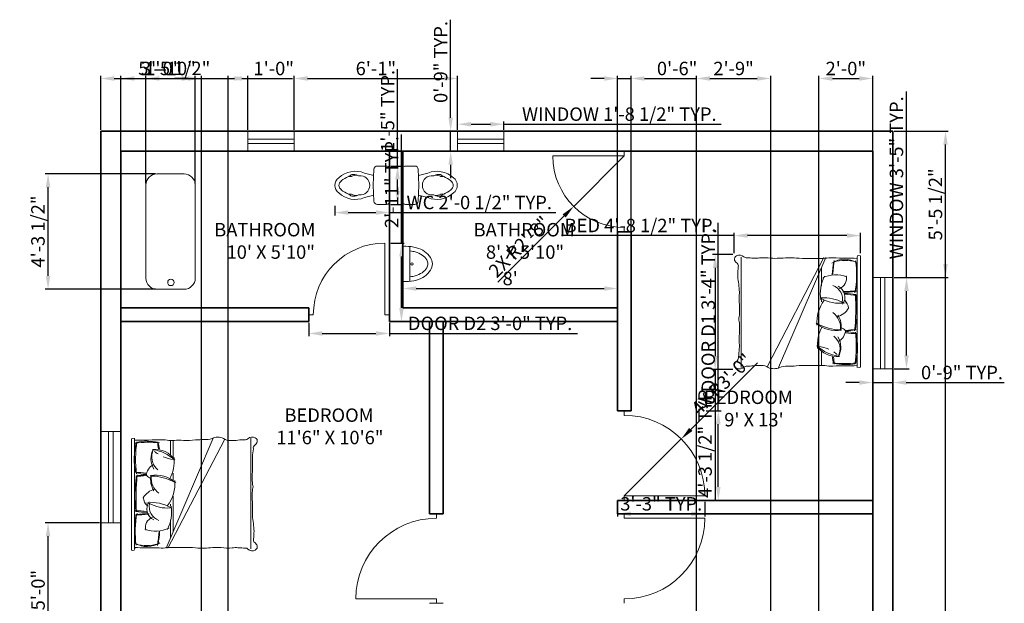
# Model space of a CAD drawing. Units: inches. Extents: x 88375 to 88815, y 24230 to 25146.
# Tile 2 of 3: x 88375 to 88815, y 24513 to 24774. Entities that reach past the tile are written whole.
import ezdxf

# ---------------------------------------------------------------- set-up
doc = ezdxf.new("R2010")
doc.units = ezdxf.units.IN
for name, color, linetype, lineweight in [('A-ANNO-DIMS', 2, 'Continuous', 18), ('A-AREA-IDEN', 7, 'Continuous', 18), ('A-WALL', 7, 'Continuous', 35), ('doors', 50, 'Continuous', 18), ('SANTEH', 5, 'Continuous', 18), ('windows', 70, 'Continuous', 18)]:
    doc.layers.add(name, color=color, linetype=linetype, lineweight=lineweight)
doc.layers.add('A-FURN', color=141, linetype='Continuous', lineweight=18, true_color=0xadddf7)
doc.styles.get("Standard").update_dxf_attribs({"font": 'arial.ttf'})
doc.dimstyles.new('ISO-25', dxfattribs={"dimtxt": 6, "dimasz": 6, "dimexe": 1.25, "dimexo": 0.625, "dimtad": 1, "dimdec": 0, "dimlunit": 3, "dimtxsty": 'Standard', "dimcen": 2.5, "dimclrd": 1, "dimclre": 1, "dimclrt": 2, "dimadec": 0, "dimazin": 0, "dimtfac": 1, "dimtdec": 0, "dimtmove": 0, "dimatfit": 3, "dimfxl": 1, "dimarcsym": 0})

# ---------------------------------------------------------------- blocks, each defined once
blk = doc.blocks.new('*D1')
at = {"layer": 'A-ANNO-DIMS', "color": 0, "lineweight": -2, "transparency": 16777216}
for p, q in [((88546.55, 24652.53), (88546.55, 24654.95)), ((88552.55, 24653.7), (88636.55, 24653.7)), ((88642.55, 24652.53), (88642.55, 24654.95))]:
    blk.add_line(p, q, dxfattribs=at)
at = {"layer": 'A-ANNO-DIMS', "color": 0, "transparency": 16777216}
for points in [[(88552.55, 24654.7), (88552.55, 24652.7), (88546.55, 24653.7)], [(88636.55, 24654.7), (88636.55, 24652.7), (88642.55, 24653.7)]]:
    blk.add_solid(points, dxfattribs=at)
at = {"layer": 'Defpoints', "color": 0, "transparency": 16777216}
for p in [(88546.55, 24651.91), (88642.55, 24653.7), (88642.55, 24651.91)]:
    blk.add_point(p, dxfattribs=at)
at = {"layer": 'A-ANNO-DIMS', "color": 0, "transparency": 16777216, "insert": (88594.55, 24657.39), "char_height": 6, "attachment_point": 5}
blk.add_mtext("8'", dxfattribs=at)
blk = doc.blocks.new('BED-DOUBLE-PLAN')
for p, q in [((1.4, 0.9), (1.4, 50.31)), ((15.52, 1.15), (36.6, 50.31)), ((16.31, 1.15), (41.56, 49.64)), ((17.42, 42.88), (17.42, 49.34)), ((18.75, 41.86), (18.75, 49.34)), ((53.33, 0.9), (53.33, 50.31)), ((18.75, 31.74), (18.75, 34.71)), ((18.75, 8.33), (18.75, 24.37)), ((17.42, 19.9), (17.42, 20.88)), ((17.42, 5.64), (17.42, 13.88))]:
    blk.add_line(p, q)
blk.add_lwpolyline([(1.54, 49.41, 0.098699), (1.25, 50.08, 0.222522), (0, 50.08), (0, 0.33, 0.171621), (1.3, 0.3, 0.102495), (1.54, 1.48, 0.015571), (6.35, 1.41, 0.00267), (12.35, 1.29, 0.058958), (15.95, 1.46, -0.038458), (19.2, 1.53, 0.025508), (23.25, 1.53, -0.039412), (28.66, 1.33, 0.016498), (32.6, 1.18, -0.035771), (40.08, 1.43, 0.045388), (45.04, 1.29, -0.080578), (47.62, 1.41, 0.026504), (50.99, 1.23, -0.211134), (52.07, 0.79, 0.329446), (55.35, 0.34, 0.37589), (56.22, 2.29, 0.123892), (55.14, 3.69, -0.342539), (54.6, 5.33, 0.07104), (54.53, 12.17, -0.036442), (54.14, 15.72, -0.046791), (54.19, 18.58, 0.023628), (54.14, 21.2, -0.055897), (54.2, 27.56, 0.053528), (54.38, 28.63, 0.053528), (54.2, 29.69, -0.055897), (54.14, 36.05, 0.026973), (54.19, 38.35, -0.036947), (54.14, 41.97, -0.036442), (54.53, 45.52, -0.281256), (55.14, 47.2, -0.521995), (55.14, 47.2, 0.123892), (56.22, 48.6, 0.37589), (55.35, 50.55, 0.329446), (52.07, 50.1, -0.211134), (50.99, 49.66, 0.026504), (47.62, 49.48, -0.06219), (44.27, 49.36, -0.218233), (41.22, 50.22, 0.123513), (38.6, 50.78, 0.129887), (36.08, 50.23, -0.095063), (32.6, 49.71, 0.016498), (28.66, 49.56, -0.039412), (23.25, 49.36, 0.025508), (19.2, 49.36, -0.038458), (15.95, 49.43, 0.058958), (12.35, 49.6, 0.00267), (6.35, 49.48, 0.015571)], format="xyb", close=True)
for centre, radius, start, end in [((28.69, 41.4), 27.41, 165.0181, 193.7392), ((7.34, -1.74), 50.25, 84.0935, 96.4707), ((54.72, 40.85), 52.84, 171.3714, 186.917), ((6.88, 26.06), 22.91, 77.3175, 101.7435), ((30.71, 48.94), 18.95, 180.6432, 190.2707), ((-1.93, 44.06), 14.51, 5.447, 17.4199), ((17.81, 41.21), 9.06, 151.6404, 211.3345), ((16.4, 41.97), 7.31, 151.8876, 231.8707), ((10.64, 34.91), 10.43, 32.3262, 97), ((7.31, 27.91), 17.47, 47.3201, 81.4624), ((20.44, 56.37), 15.6, 229.9508, 236.951), ((20.44, 56.37), 15.6, 246.2982, 263.8539), ((2.46, 40.16), 16.73, 330.9467, 5.467), ((12.85, 33.14), 6.24, 118.1996, 176.5061), ((56.67, 24.77), 55.1, 170.934, 187.4266), ((2.85, 15.46), 19.59, 79.1667, 93.123), ((2.68, 52.73), 19.37, 267.8261, 281.4767), ((6.96, 53.59), 19.33, 255.3434, 268.3876), ((106.24, 23.67), 104.16, 174.3658, 183.3969), ((7.12, 7.71), 26.2, 91.8337, 100.6945), ((8.83, 34.94), 2.36, 210.1134, 265.8974), ((10.93, 20.25), 13.55, 49.1339, 100.5299), ((18.11, 31.85), 9.49, 168.4081, 212.0077), ((17.21, 32.51), 8.35, 173.5607, 234.2853), ((8.19, 10.11), 23.35, 61.605, 88.1749), ((2.96, 30.11), 16.53, 323.2201, 4.4972), ((12.63, 19.42), 8.48, 105.4018, 149.7122), ((11.01, 24.39), 5.75, 186.8992, 226.0421), ((2.41, -6.96), 24.84, 79.589, 92.0447), ((6.97, 44.4), 27.2, 259.5301, 269.934), ((9.41, 5.14), 16.41, 58.6542, 99.1977), ((12.4, 18.76), 5.47, 144.1671, 243.8421), ((16.24, 36.43), 17.32, 241.0456, 274.1497), ((14.48, 19.78), 6.53, 168.0413, 250.8342), ((1.41, 17.17), 16.55, 332.3859, 9.8951), ((35.22, 9.22), 33.81, 168.0142, 190.5125), ((43.42, 8.57), 41.72, 168.5485, 188.3029), ((1.64, 92.63), 76.52, 270.1063, 274.3312), ((7.34, -22.96), 39.54, 89.1536, 97.5533), ((10.98, 10.47), 4.74, 108.9387, 194.6725), ((10.84, 22.26), 13.47, 249.3026, 296.5026), ((274.44, -22.62), 263.89, 173.2132, 174.5476), ((-20.26, 9.91), 32.87, 348.1169, 357.8849), ((7.08, 12.11), 10.21, 237.51, 303.8336), ((6.79, 19.75), 17.39, 253.9263, 287.1409)]:
    blk.add_arc(centre, radius, start, end)
blk = doc.blocks.new('WC-CISTERN-PLAN')
at = {"ltscale": 20}
for p, q in [((17.36, 12.87), (13.25, 13.99)), ((17.16, 8.57), (17.48, 15.67)), ((23.09, 17.14), (19.01, 17.14)), ((24.36, 0.67), (24.36, 16.47)), ((6.41, 12.48), (7.47, 12.48)), ((6.55, 12.64), (7.12, 13.12)), ((6.41, 4.52), (7.47, 4.52)), ((17.16, 8.57), (17.48, 1.46)), ((6.55, 4.36), (7.12, 3.88)), ((17.36, 4.13), (13.25, 3.01)), ((23.09, 0), (19.01, 0))]:
    blk.add_line(p, q, dxfattribs=at)
for centre, radius, start, end in [((9.17, 3.81), 10.97, 68.2076, 132.5865), ((7.71, 12.42), 0.912, 100.6032, 130), ((8.29, 9.29), 4.1, 61.4258, 100.6032), ((19.01, 15.6), 1.53, 90, 177.4245), ((23.09, 15.47), 1.66, 43.4731, 90), ((24.15, 16.47), 0.215, 0, 43.4731), ((4.15, 8.5), 4.15, 125.2885, 180), ((4.15, 8.5), 2.32, 122.7026, 180), ((9.17, 3.81), 9.15, 109.6249, 133.388), ((6.41, 11.56), 0.912, 90, 109.6249), ((5.96, 13.34), 0.912, 288.6119, 310), ((9.88, 7.58), 5.47, 89.5478, 116.498), ((10.69, 13.69), 0.912, 241.4258, 276.6477), ((11.3, 8.5), 4.31, 0, 96.6477), ((4.15, 8.5), 4.15, 180, 234.7115), ((9.17, 13.19), 10.97, 227.4135, 291.7924), ((4.15, 8.5), 2.32, 180, 237.2974), ((9.17, 13.19), 9.15, 226.612, 250.3751), ((6.41, 5.43), 0.912, 250.3751, 270), ((5.96, 3.66), 0.912, 50, 71.3881), ((9.88, 9.42), 5.47, 243.502, 270.4522), ((11.3, 8.5), 4.31, 263.3523, 0), ((7.71, 4.58), 0.912, 230, 259.3968), ((8.29, 7.71), 4.1, 259.3968, 298.5742), ((10.69, 3.31), 0.912, 83.3523, 118.5742), ((19.01, 1.53), 1.53, 182.5755, 270), ((23.09, 1.66), 1.66, 270, 316.5269), ((24.15, 0.67), 0.215, 316.5269, 0)]:
    blk.add_arc(centre, radius, start, end, dxfattribs=at)
blk = doc.blocks.new('WINDOW-PLAN-WIDE')
for p, q in [((3.5, 40.79), (3.5, 0)), ((5.5, 40.79), (5.5, 0))]:
    blk.add_line(p, q)
blk.add_lwpolyline([(0, 0), (9, 0), (9, 40.79), (0, 40.79)], close=True)
blk = doc.blocks.new('WINDOW-PLAN-NARROW')
for p, q in [((0, 5.5), (20.7, 5.5)), ((0, 3.5), (20.7, 3.5)), ((0, 0), (6, 0))]:
    blk.add_line(p, q)
blk.add_lwpolyline([(0, 0), (20.7, 0), (20.7, 9), (0, 9)], close=True)
blk = doc.blocks.new('DOOR-SWING-32IN')
for p, q in [((34, 3), (34, 35)), ((36, 6), (36, 0)), ((2, 3), (0, 3)), ((36, 3), (34, 3))]:
    blk.add_line(p, q)
blk.add_arc((34, 3), 32, 90, 180)
blk = doc.blocks.new('DOOR-SWING-36IN')
for p, q in [((3, 38), (3, 40)), ((3, 0), (3, 2)), ((3, 2), (39, 2)), ((6, 0), (0, 0))]:
    blk.add_line(p, q)
blk.add_arc((3, 2), 36, 0, 90)
blk = doc.blocks.new('*D17')
at = {"layer": 'A-ANNO-DIMS', "color": 1, "lineweight": -2, "transparency": 16777216}
for p, q in [((88771.67, 24658.59), (88771.67, 24741.77)), ((88766.18, 24658.59), (88772.92, 24658.59)), ((88771.67, 24623.81), (88771.67, 24652.59)), ((88766.18, 24617.81), (88772.92, 24617.81))]:
    blk.add_line(p, q, dxfattribs=at)
at = {"layer": 'A-ANNO-DIMS', "color": 1, "transparency": 16777216}
for points in [[(88770.67, 24652.59), (88772.67, 24652.59), (88771.67, 24658.59)], [(88770.67, 24623.81), (88772.67, 24623.81), (88771.67, 24617.81)]]:
    blk.add_solid(points, dxfattribs=at)
at = {"layer": 'Defpoints', "color": 0, "transparency": 16777216}
for p in [(88765.55, 24658.59), (88771.67, 24658.59), (88765.55, 24617.81)]:
    blk.add_point(p, dxfattribs=at)
at = {"layer": 'A-ANNO-DIMS', "color": 2, "transparency": 16777216, "insert": (88767.94, 24703.18), "char_height": 6, "attachment_point": 5, "rotation": 90}
blk.add_mtext('WINDOW 3\'-5" TYP.', dxfattribs=at)
blk = doc.blocks.new('*D18')
at = {"layer": 'A-ANNO-DIMS', "color": 1, "lineweight": -2, "transparency": 16777216}
for p, q in [((88756.55, 24617.18), (88756.55, 24610.44)), ((88765.55, 24617.18), (88765.55, 24610.44)), ((88750.55, 24611.69), (88744.55, 24611.69)), ((88756.55, 24611.69), (88765.55, 24611.69)), ((88771.55, 24611.69), (88815.38, 24611.69))]:
    blk.add_line(p, q, dxfattribs=at)
at = {"layer": 'A-ANNO-DIMS', "color": 1, "transparency": 16777216}
for points in [[(88750.55, 24612.69), (88750.55, 24610.69), (88756.55, 24611.69)], [(88771.55, 24612.69), (88771.55, 24610.69), (88765.55, 24611.69)]]:
    blk.add_solid(points, dxfattribs=at)
at = {"layer": 'Defpoints', "color": 0, "transparency": 16777216}
for p in [(88756.55, 24617.81), (88765.55, 24617.81), (88765.55, 24611.69)]:
    blk.add_point(p, dxfattribs=at)
at = {"layer": 'A-ANNO-DIMS', "color": 2, "transparency": 16777216, "insert": (88796.46, 24615.38), "char_height": 6, "attachment_point": 5}
blk.add_mtext('0\'-9" TYP.', dxfattribs=at)
blk = doc.blocks.new('*D19')
at = {"layer": 'A-ANNO-DIMS', "color": 1, "lineweight": -2, "transparency": 16777216}
for p, q in [((88687.55, 24599.02), (88687.55, 24683.07)), ((88682.18, 24599.02), (88688.8, 24599.02)), ((88687.55, 24565.02), (88687.55, 24593.02)), ((88682.18, 24559.02), (88688.8, 24559.02))]:
    blk.add_line(p, q, dxfattribs=at)
at = {"layer": 'A-ANNO-DIMS', "color": 1, "transparency": 16777216}
for points in [[(88686.55, 24593.02), (88688.55, 24593.02), (88687.55, 24599.02)], [(88686.55, 24565.02), (88688.55, 24565.02), (88687.55, 24559.02)]]:
    blk.add_solid(points, dxfattribs=at)
at = {"layer": 'Defpoints', "color": 0, "transparency": 16777216}
for p in [(88681.55, 24599.02), (88687.55, 24599.02), (88681.55, 24559.02)]:
    blk.add_point(p, dxfattribs=at)
at = {"layer": 'A-ANNO-DIMS', "color": 2, "transparency": 16777216, "insert": (88683.82, 24644.05), "char_height": 6, "attachment_point": 5, "rotation": 90}
blk.add_mtext('DOOR D1 3\'-4" TYP.', dxfattribs=at)
blk = doc.blocks.new('*D20')
at = {"layer": 'A-ANNO-DIMS', "color": 1, "lineweight": -2, "transparency": 16777216}
for p, q in [((88642.55, 24558.4), (88642.55, 24551.77)), ((88681.55, 24558.4), (88681.55, 24551.77)), ((88648.55, 24553.02), (88675.55, 24553.02))]:
    blk.add_line(p, q, dxfattribs=at)
at = {"layer": 'A-ANNO-DIMS', "color": 1, "transparency": 16777216}
for points in [[(88648.55, 24554.02), (88648.55, 24552.02), (88642.55, 24553.02)], [(88675.55, 24554.02), (88675.55, 24552.02), (88681.55, 24553.02)]]:
    blk.add_solid(points, dxfattribs=at)
at = {"layer": 'Defpoints', "color": 0, "transparency": 16777216}
for p in [(88642.55, 24559.02), (88681.55, 24559.02), (88681.55, 24553.02)]:
    blk.add_point(p, dxfattribs=at)
at = {"layer": 'A-ANNO-DIMS', "color": 2, "transparency": 16777216, "insert": (88662.05, 24556.71), "char_height": 6, "attachment_point": 5}
blk.add_mtext('3\'-3" TYP.', dxfattribs=at)
blk = doc.blocks.new('*D21')
at = {"layer": 'A-ANNO-DIMS', "color": 1, "lineweight": -2, "transparency": 16777216}
for p, q in [((88694.61, 24669.53), (88694.61, 24678.62)), ((88751.07, 24669.53), (88751.07, 24678.62)), ((88694.61, 24677.37), (88617.51, 24677.37)), ((88745.07, 24677.37), (88700.61, 24677.37))]:
    blk.add_line(p, q, dxfattribs=at)
at = {"layer": 'A-ANNO-DIMS', "color": 1, "transparency": 16777216}
for points in [[(88700.61, 24678.37), (88700.61, 24676.37), (88694.61, 24677.37)], [(88745.07, 24678.37), (88745.07, 24676.37), (88751.07, 24677.37)]]:
    blk.add_solid(points, dxfattribs=at)
at = {"layer": 'Defpoints', "color": 0, "transparency": 16777216}
for p in [(88694.61, 24677.37), (88694.61, 24668.9), (88751.07, 24668.9)]:
    blk.add_point(p, dxfattribs=at)
at = {"layer": 'A-ANNO-DIMS', "color": 2, "transparency": 16777216, "insert": (88653.06, 24681.1), "char_height": 6, "attachment_point": 5}
blk.add_mtext('BED 4\'-8 1/2" TYP.', dxfattribs=at)
blk = doc.blocks.new('*D22')
at = {"layer": 'A-ANNO-DIMS', "color": 1, "lineweight": -2, "transparency": 16777216}
for p, q in [((88693.98, 24668.9), (88684.89, 24668.9)), ((88686.14, 24662.9), (88686.14, 24623.52)), ((88693.98, 24617.52), (88684.89, 24617.52)), ((88686.14, 24617.52), (88686.14, 24559.48))]:
    blk.add_line(p, q, dxfattribs=at)
at = {"layer": 'A-ANNO-DIMS', "color": 1, "transparency": 16777216}
for points in [[(88685.14, 24662.9), (88687.14, 24662.9), (88686.14, 24668.9)], [(88685.14, 24623.52), (88687.14, 24623.52), (88686.14, 24617.52)]]:
    blk.add_solid(points, dxfattribs=at)
at = {"layer": 'Defpoints', "color": 0, "transparency": 16777216}
for p in [(88694.61, 24668.9), (88686.14, 24617.52), (88694.61, 24617.52)]:
    blk.add_point(p, dxfattribs=at)
at = {"layer": 'A-ANNO-DIMS', "color": 2, "transparency": 16777216, "insert": (88682.41, 24585.5), "char_height": 6, "attachment_point": 5, "rotation": 90}
blk.add_mtext('4\'-3 1/2" TYP.', dxfattribs=at)
blk = doc.blocks.new('*D25')
at = {"layer": 'A-ANNO-DIMS', "color": 1, "lineweight": -2, "transparency": 16777216}
for p, q in [((88516.19, 24690.68), (88516.19, 24686.4)), ((88522.19, 24687.65), (88534.55, 24687.65)), ((88540.55, 24690.68), (88540.55, 24686.4)), ((88540.55, 24687.65), (88614.9, 24687.65))]:
    blk.add_line(p, q, dxfattribs=at)
at = {"layer": 'A-ANNO-DIMS', "color": 1, "transparency": 16777216}
for points in [[(88522.19, 24688.65), (88522.19, 24686.65), (88516.19, 24687.65)], [(88534.55, 24688.65), (88534.55, 24686.65), (88540.55, 24687.65)]]:
    blk.add_solid(points, dxfattribs=at)
at = {"layer": 'Defpoints', "color": 0, "transparency": 16777216}
for p in [(88516.19, 24691.31), (88540.55, 24691.31), (88540.55, 24687.65)]:
    blk.add_point(p, dxfattribs=at)
at = {"layer": 'A-ANNO-DIMS', "color": 2, "transparency": 16777216, "insert": (88580.72, 24691.38), "char_height": 6, "attachment_point": 5}
blk.add_mtext('WC 2\'-0 1/2" TYP.', dxfattribs=at)
blk = doc.blocks.new('*D26')
at = {"layer": 'A-ANNO-DIMS', "color": 1, "lineweight": -2, "transparency": 16777216}
for p, q in [((88544.21, 24708.44), (88544.21, 24751.7)), ((88541.18, 24708.44), (88545.46, 24708.44)), ((88544.21, 24697.31), (88544.21, 24702.44)), ((88541.18, 24691.31), (88545.46, 24691.31))]:
    blk.add_line(p, q, dxfattribs=at)
at = {"layer": 'A-ANNO-DIMS', "color": 1, "transparency": 16777216}
for points in [[(88543.21, 24702.44), (88545.21, 24702.44), (88544.21, 24708.44)], [(88543.21, 24697.31), (88545.21, 24697.31), (88544.21, 24691.31)]]:
    blk.add_solid(points, dxfattribs=at)
at = {"layer": 'Defpoints', "color": 0, "transparency": 16777216}
for p in [(88540.55, 24708.44), (88544.21, 24708.44), (88540.55, 24691.31)]:
    blk.add_point(p, dxfattribs=at)
at = {"layer": 'A-ANNO-DIMS', "color": 2, "transparency": 16777216, "insert": (88540.52, 24733.07), "char_height": 6, "attachment_point": 5, "rotation": 90}
blk.add_mtext('1\'-5" TYP.', dxfattribs=at)
blk = doc.blocks.new('*D29')
at = {"layer": 'A-ANNO-DIMS', "color": 1, "lineweight": -2, "transparency": 16777216}
for p, q in [((88571.04, 24724.65), (88571.04, 24728.38)), ((88577.04, 24727.13), (88585.73, 24727.13)), ((88591.73, 24724.65), (88591.73, 24728.38)), ((88591.73, 24727.13), (88688.89, 24727.13))]:
    blk.add_line(p, q, dxfattribs=at)
at = {"layer": 'A-ANNO-DIMS', "color": 1, "transparency": 16777216}
for points in [[(88577.04, 24728.13), (88577.04, 24726.13), (88571.04, 24727.13)], [(88585.73, 24728.13), (88585.73, 24726.13), (88591.73, 24727.13)]]:
    blk.add_solid(points, dxfattribs=at)
at = {"layer": 'Defpoints', "color": 0, "transparency": 16777216}
for p in [(88591.73, 24727.13), (88571.04, 24724.02), (88591.73, 24724.02)]:
    blk.add_point(p, dxfattribs=at)
at = {"layer": 'A-ANNO-DIMS', "color": 2, "transparency": 16777216, "insert": (88643.31, 24730.86), "char_height": 6, "attachment_point": 5}
blk.add_mtext('WINDOW 1\'-8 1/2" TYP.', dxfattribs=at)
blk = doc.blocks.new('*D30')
at = {"layer": 'A-ANNO-DIMS', "color": 1, "lineweight": -2, "transparency": 16777216}
for p, q in [((88567.93, 24730.02), (88567.93, 24773.85)), ((88570.41, 24724.02), (88566.68, 24724.02)), ((88567.93, 24715.02), (88567.93, 24724.02)), ((88570.41, 24715.02), (88566.68, 24715.02)), ((88567.93, 24709.02), (88567.93, 24703.02))]:
    blk.add_line(p, q, dxfattribs=at)
at = {"layer": 'A-ANNO-DIMS', "color": 1, "transparency": 16777216}
for points in [[(88566.93, 24730.02), (88568.93, 24730.02), (88567.93, 24724.02)], [(88566.93, 24709.02), (88568.93, 24709.02), (88567.93, 24715.02)]]:
    blk.add_solid(points, dxfattribs=at)
at = {"layer": 'Defpoints', "color": 0, "transparency": 16777216}
for p in [(88567.93, 24724.02), (88571.04, 24724.02), (88571.04, 24715.02)]:
    blk.add_point(p, dxfattribs=at)
at = {"layer": 'A-ANNO-DIMS', "color": 2, "transparency": 16777216, "insert": (88564.24, 24754.94), "char_height": 6, "attachment_point": 5, "rotation": 90}
blk.add_mtext('0\'-9" TYP.', dxfattribs=at)
blk = doc.blocks.new('*D31')
at = {"layer": 'A-ANNO-DIMS', "color": 1, "lineweight": -2, "transparency": 16777216}
for p, q in [((88504.55, 24638.4), (88504.55, 24632.37)), ((88540.55, 24638.4), (88540.55, 24632.37)), ((88510.55, 24633.62), (88534.55, 24633.62)), ((88540.55, 24633.62), (88624.6, 24633.62))]:
    blk.add_line(p, q, dxfattribs=at)
at = {"layer": 'A-ANNO-DIMS', "color": 1, "transparency": 16777216}
for points in [[(88510.55, 24634.62), (88510.55, 24632.62), (88504.55, 24633.62)], [(88534.55, 24634.62), (88534.55, 24632.62), (88540.55, 24633.62)]]:
    blk.add_solid(points, dxfattribs=at)
at = {"layer": 'Defpoints', "color": 0, "transparency": 16777216}
for p in [(88504.55, 24639.02), (88540.55, 24639.02), (88540.55, 24633.62)]:
    blk.add_point(p, dxfattribs=at)
at = {"layer": 'A-ANNO-DIMS', "color": 2, "transparency": 16777216, "insert": (88585.57, 24637.36), "char_height": 6, "attachment_point": 5}
blk.add_mtext('DOOR D2 3\'-0" TYP.', dxfattribs=at)
blk = doc.blocks.new('*D32')
at = {"layer": 'A-ANNO-DIMS', "color": 1, "lineweight": -2, "transparency": 16777216}
for p, q in [((88545.95, 24674.02), (88545.95, 24722.61)), ((88541.18, 24674.02), (88547.2, 24674.02)), ((88545.95, 24645.02), (88545.95, 24668.02)), ((88541.18, 24639.02), (88547.2, 24639.02))]:
    blk.add_line(p, q, dxfattribs=at)
at = {"layer": 'A-ANNO-DIMS', "color": 1, "transparency": 16777216}
for points in [[(88544.95, 24668.02), (88546.95, 24668.02), (88545.95, 24674.02)], [(88544.95, 24645.02), (88546.95, 24645.02), (88545.95, 24639.02)]]:
    blk.add_solid(points, dxfattribs=at)
at = {"layer": 'Defpoints', "color": 0, "transparency": 16777216}
for p in [(88540.55, 24674.02), (88545.95, 24674.02), (88540.55, 24639.02)]:
    blk.add_point(p, dxfattribs=at)
at = {"layer": 'A-ANNO-DIMS', "color": 2, "transparency": 16777216, "insert": (88542.31, 24701.32), "char_height": 6, "attachment_point": 5, "rotation": 90}
blk.add_mtext('2\'-11" TYP.', dxfattribs=at)
blk = doc.blocks.new('*D34')
at = {"layer": 'A-ANNO-DIMS', "color": 1, "lineweight": -2, "transparency": 16777216}
for p, q in [((88766.18, 24724.02), (88790.35, 24724.02)), ((88789.1, 24261.02), (88789.1, 24718.02)), ((88766.18, 24255.02), (88790.35, 24255.02))]:
    blk.add_line(p, q, dxfattribs=at)
at = {"layer": 'A-ANNO-DIMS', "color": 1, "transparency": 16777216}
for points in [[(88788.1, 24718.02), (88790.1, 24718.02), (88789.1, 24724.02)], [(88788.1, 24261.02), (88790.1, 24261.02), (88789.1, 24255.02)]]:
    blk.add_solid(points, dxfattribs=at)
at = {"layer": 'Defpoints', "color": 0, "transparency": 16777216}
for p in [(88765.55, 24724.02), (88789.1, 24724.02), (88765.55, 24255.02)]:
    blk.add_point(p, dxfattribs=at)
at = {"layer": 'A-ANNO-DIMS', "color": 2, "transparency": 16777216, "insert": (88785.41, 24489.52), "char_height": 6, "attachment_point": 5, "rotation": 90}
blk.add_mtext('39\'-1"', dxfattribs=at)
blk = doc.blocks.new('*D35')
at = {"layer": 'A-ANNO-DIMS', "color": 1, "lineweight": -2, "transparency": 16777216}
for p, q in [((88411.55, 24724.65), (88411.55, 24748.82)), ((88477.28, 24724.65), (88477.28, 24748.82)), ((88417.55, 24747.57), (88471.28, 24747.57))]:
    blk.add_line(p, q, dxfattribs=at)
at = {"layer": 'A-ANNO-DIMS', "color": 1, "transparency": 16777216}
for points in [[(88417.55, 24748.57), (88417.55, 24746.57), (88411.55, 24747.57)], [(88471.28, 24748.57), (88471.28, 24746.57), (88477.28, 24747.57)]]:
    blk.add_solid(points, dxfattribs=at)
at = {"layer": 'Defpoints', "color": 0, "transparency": 16777216}
for p in [(88477.28, 24747.57), (88411.55, 24724.02), (88477.28, 24724.02)]:
    blk.add_point(p, dxfattribs=at)
at = {"layer": 'A-ANNO-DIMS', "color": 2, "transparency": 16777216, "insert": (88444.42, 24751.3), "char_height": 6, "attachment_point": 5}
blk.add_mtext('5\'-5 1/2"', dxfattribs=at)
blk = doc.blocks.new('*D36')
at = {"layer": 'A-ANNO-DIMS', "color": 1, "lineweight": -2, "transparency": 16777216}
for p, q in [((88497.98, 24724.65), (88497.98, 24748.82)), ((88571.04, 24724.65), (88571.04, 24748.82)), ((88503.98, 24747.57), (88565.04, 24747.57))]:
    blk.add_line(p, q, dxfattribs=at)
at = {"layer": 'A-ANNO-DIMS', "color": 1, "transparency": 16777216}
for points in [[(88503.98, 24748.57), (88503.98, 24746.57), (88497.98, 24747.57)], [(88565.04, 24748.57), (88565.04, 24746.57), (88571.04, 24747.57)]]:
    blk.add_solid(points, dxfattribs=at)
at = {"layer": 'Defpoints', "color": 0, "transparency": 16777216}
for p in [(88571.04, 24747.57), (88497.98, 24724.02), (88571.04, 24724.02)]:
    blk.add_point(p, dxfattribs=at)
at = {"layer": 'A-ANNO-DIMS', "color": 2, "transparency": 16777216, "insert": (88534.51, 24751.26), "char_height": 6, "attachment_point": 5}
blk.add_mtext('6\'-1"', dxfattribs=at)
blk = doc.blocks.new('*D38')
at = {"layer": 'A-ANNO-DIMS', "color": 1, "lineweight": -2, "transparency": 16777216}
for p, q in [((88766.18, 24724.02), (88790.35, 24724.02)), ((88789.1, 24664.59), (88789.1, 24718.02)), ((88766.18, 24658.59), (88790.35, 24658.59))]:
    blk.add_line(p, q, dxfattribs=at)
at = {"layer": 'A-ANNO-DIMS', "color": 1, "transparency": 16777216}
for points in [[(88788.1, 24718.02), (88790.1, 24718.02), (88789.1, 24724.02)], [(88788.1, 24664.59), (88790.1, 24664.59), (88789.1, 24658.59)]]:
    blk.add_solid(points, dxfattribs=at)
at = {"layer": 'Defpoints', "color": 0, "transparency": 16777216}
for p in [(88765.55, 24724.02), (88789.1, 24724.02), (88765.55, 24658.59)]:
    blk.add_point(p, dxfattribs=at)
at = {"layer": 'A-ANNO-DIMS', "color": 2, "transparency": 16777216, "insert": (88785.38, 24691.31), "char_height": 6, "attachment_point": 5, "rotation": 90}
blk.add_mtext('5\'-5 1/2"', dxfattribs=at)
blk = doc.blocks.new('*D41')
at = {"layer": 'A-ANNO-DIMS', "color": 1, "lineweight": -2, "transparency": 16777216}
for p, q in [((88410.93, 24549.01), (88386.75, 24549.01)), ((88388, 24494.84), (88388, 24543.01)), ((88410.93, 24488.84), (88386.75, 24488.84))]:
    blk.add_line(p, q, dxfattribs=at)
at = {"layer": 'A-ANNO-DIMS', "color": 1, "transparency": 16777216}
for points in [[(88387, 24543.01), (88389, 24543.01), (88388, 24549.01)], [(88387, 24494.84), (88389, 24494.84), (88388, 24488.84)]]:
    blk.add_solid(points, dxfattribs=at)
at = {"layer": 'Defpoints', "color": 0, "transparency": 16777216}
for p in [(88388, 24549.01), (88411.55, 24549.01), (88411.55, 24488.84)]:
    blk.add_point(p, dxfattribs=at)
at = {"layer": 'A-ANNO-DIMS', "color": 2, "transparency": 16777216, "insert": (88384.31, 24518.92), "char_height": 6, "attachment_point": 5, "rotation": 90}
blk.add_mtext('5\'-0"', dxfattribs=at)
blk = doc.blocks.new('*D43')
at = {"layer": 'A-ANNO-DIMS', "color": 1, "lineweight": -2, "transparency": 16777216}
for p, q in [((88420.55, 24345.65), (88420.55, 24748.82)), ((88456.55, 24345.65), (88456.55, 24748.82)), ((88426.55, 24747.57), (88450.55, 24747.57))]:
    blk.add_line(p, q, dxfattribs=at)
at = {"layer": 'A-ANNO-DIMS', "color": 1, "transparency": 16777216}
for points in [[(88426.55, 24748.57), (88426.55, 24746.57), (88420.55, 24747.57)], [(88450.55, 24748.57), (88450.55, 24746.57), (88456.55, 24747.57)]]:
    blk.add_solid(points, dxfattribs=at)
at = {"layer": 'Defpoints', "color": 0, "transparency": 16777216}
for p in [(88456.55, 24747.57), (88420.55, 24345.02), (88456.55, 24345.02)]:
    blk.add_point(p, dxfattribs=at)
at = {"layer": 'A-ANNO-DIMS', "color": 2, "transparency": 16777216, "insert": (88438.55, 24751.26), "char_height": 6, "attachment_point": 5}
blk.add_mtext('3\'-0"', dxfattribs=at)
blk = doc.blocks.new('*D45')
at = {"layer": 'A-ANNO-DIMS', "color": 1, "lineweight": -2, "transparency": 16777216}
for p, q in [((88456.55, 24417.65), (88456.55, 24748.82)), ((88468.55, 24417.65), (88468.55, 24748.82)), ((88450.55, 24747.57), (88444.55, 24747.57)), ((88456.55, 24747.57), (88468.55, 24747.57)), ((88474.55, 24747.57), (88497.19, 24747.57))]:
    blk.add_line(p, q, dxfattribs=at)
at = {"layer": 'A-ANNO-DIMS', "color": 1, "transparency": 16777216}
for points in [[(88450.55, 24748.57), (88450.55, 24746.57), (88456.55, 24747.57)], [(88474.55, 24748.57), (88474.55, 24746.57), (88468.55, 24747.57)]]:
    blk.add_solid(points, dxfattribs=at)
at = {"layer": 'Defpoints', "color": 0, "transparency": 16777216}
for p in [(88468.55, 24747.57), (88456.55, 24417.02), (88468.55, 24417.02)]:
    blk.add_point(p, dxfattribs=at)
at = {"layer": 'A-ANNO-DIMS', "color": 2, "transparency": 16777216, "insert": (88488.87, 24751.26), "char_height": 6, "attachment_point": 5}
blk.add_mtext('1\'-0"', dxfattribs=at)
blk = doc.blocks.new('*D46')
at = {"layer": 'A-ANNO-DIMS', "color": 1, "lineweight": -2, "transparency": 16777216}
for p, q in [((88642.55, 24599.65), (88642.55, 24748.82)), ((88648.55, 24599.65), (88648.55, 24748.82)), ((88636.55, 24747.57), (88630.55, 24747.57)), ((88642.55, 24747.57), (88648.55, 24747.57)), ((88654.55, 24747.57), (88677.75, 24747.57))]:
    blk.add_line(p, q, dxfattribs=at)
at = {"layer": 'A-ANNO-DIMS', "color": 1, "transparency": 16777216}
for points in [[(88636.55, 24748.57), (88636.55, 24746.57), (88642.55, 24747.57)], [(88654.55, 24748.57), (88654.55, 24746.57), (88648.55, 24747.57)]]:
    blk.add_solid(points, dxfattribs=at)
at = {"layer": 'Defpoints', "color": 0, "transparency": 16777216}
for p in [(88648.55, 24747.57), (88642.55, 24599.02), (88648.55, 24599.02)]:
    blk.add_point(p, dxfattribs=at)
at = {"layer": 'A-ANNO-DIMS', "color": 2, "transparency": 16777216, "insert": (88669.15, 24751.26), "char_height": 6, "attachment_point": 5}
blk.add_mtext('0\'-6"', dxfattribs=at)
blk = doc.blocks.new('*D47')
at = {"layer": 'A-ANNO-DIMS', "color": 1, "lineweight": -2, "transparency": 16777216}
for p, q in [((88732.55, 24361.84), (88732.55, 24748.82)), ((88756.55, 24361.84), (88756.55, 24748.82)), ((88738.55, 24747.57), (88750.55, 24747.57))]:
    blk.add_line(p, q, dxfattribs=at)
at = {"layer": 'A-ANNO-DIMS', "color": 1, "transparency": 16777216}
for points in [[(88738.55, 24748.57), (88738.55, 24746.57), (88732.55, 24747.57)], [(88750.55, 24748.57), (88750.55, 24746.57), (88756.55, 24747.57)]]:
    blk.add_solid(points, dxfattribs=at)
at = {"layer": 'Defpoints', "color": 0, "transparency": 16777216}
for p in [(88756.55, 24747.57), (88732.55, 24361.22), (88756.55, 24361.22)]:
    blk.add_point(p, dxfattribs=at)
at = {"layer": 'A-ANNO-DIMS', "color": 2, "transparency": 16777216, "insert": (88744.55, 24751.26), "char_height": 6, "attachment_point": 5}
blk.add_mtext('2\'-0"', dxfattribs=at)
blk = doc.blocks.new('*D50')
at = {"layer": 'A-ANNO-DIMS', "color": 1, "lineweight": -2, "transparency": 16777216}
for p, q in [((88677.79, 24271.69), (88677.79, 24748.82)), ((88710.98, 24271.69), (88710.98, 24748.82)), ((88683.79, 24747.57), (88704.98, 24747.57))]:
    blk.add_line(p, q, dxfattribs=at)
at = {"layer": 'A-ANNO-DIMS', "color": 1, "transparency": 16777216}
for points in [[(88683.79, 24748.57), (88683.79, 24746.57), (88677.79, 24747.57)], [(88704.98, 24748.57), (88704.98, 24746.57), (88710.98, 24747.57)]]:
    blk.add_solid(points, dxfattribs=at)
at = {"layer": 'Defpoints', "color": 0, "transparency": 16777216}
for p in [(88710.98, 24747.57), (88677.79, 24271.06), (88710.98, 24271.06)]:
    blk.add_point(p, dxfattribs=at)
at = {"layer": 'A-ANNO-DIMS', "color": 2, "transparency": 16777216, "insert": (88694.38, 24751.26), "char_height": 6, "attachment_point": 5}
blk.add_mtext('2\'-9"', dxfattribs=at)
blk = doc.blocks.new('*D52')
at = {"layer": 'A-ANNO-DIMS', "color": 1, "lineweight": -2, "transparency": 16777216}
for p, q in [((88431.69, 24700.6), (88431.69, 24748.82)), ((88453.78, 24700.6), (88453.78, 24748.82)), ((88437.69, 24747.57), (88447.78, 24747.57))]:
    blk.add_line(p, q, dxfattribs=at)
at = {"layer": 'A-ANNO-DIMS', "color": 1, "transparency": 16777216}
for points in [[(88437.69, 24748.57), (88437.69, 24746.57), (88431.69, 24747.57)], [(88447.78, 24748.57), (88447.78, 24746.57), (88453.78, 24747.57)]]:
    blk.add_solid(points, dxfattribs=at)
at = {"layer": 'Defpoints', "color": 0, "transparency": 16777216}
for p in [(88453.78, 24747.57), (88431.69, 24699.98), (88453.78, 24699.98)]:
    blk.add_point(p, dxfattribs=at)
at = {"layer": 'A-ANNO-DIMS', "color": 2, "transparency": 16777216, "insert": (88442.73, 24751.26), "char_height": 6, "attachment_point": 5}
blk.add_mtext('1\'-10"', dxfattribs=at)
blk = doc.blocks.new('*D53')
at = {"layer": 'A-ANNO-DIMS', "color": 1, "lineweight": -2, "transparency": 16777216}
for p, q in [((88436.06, 24704.98), (88386.75, 24704.98)), ((88388, 24659.37), (88388, 24698.98)), ((88436.06, 24653.37), (88386.75, 24653.37))]:
    blk.add_line(p, q, dxfattribs=at)
at = {"layer": 'A-ANNO-DIMS', "color": 1, "transparency": 16777216}
for points in [[(88387, 24698.98), (88389, 24698.98), (88388, 24704.98)], [(88387, 24659.37), (88389, 24659.37), (88388, 24653.37)]]:
    blk.add_solid(points, dxfattribs=at)
at = {"layer": 'Defpoints', "color": 0, "transparency": 16777216}
for p in [(88388, 24704.98), (88436.69, 24704.98), (88436.69, 24653.37)]:
    blk.add_point(p, dxfattribs=at)
at = {"layer": 'A-ANNO-DIMS', "color": 2, "transparency": 16777216, "insert": (88384.27, 24679.18), "char_height": 6, "attachment_point": 5, "rotation": 90}
blk.add_mtext('4\'-3 1/2"', dxfattribs=at)
blk = doc.blocks.new('*D66')
at = {"layer": 'A-ANNO-DIMS', "color": 1, "lineweight": -2, "transparency": 16777216}
for p, q in [((88705, 24620.47), (88675.25, 24590.72)), ((88645.55, 24561.02), (88671.01, 24586.48))]:
    blk.add_line(p, q, dxfattribs=at)
at = {"layer": 'A-ANNO-DIMS', "color": 1, "transparency": 16777216}
blk.add_solid([(88674.54, 24591.43), (88675.96, 24590.02), (88671.01, 24586.48)], dxfattribs=at)
at = {"layer": 'Defpoints', "color": 0, "transparency": 16777216}
for p in [(88671.01, 24586.48), (88645.55, 24561.02)]:
    blk.add_point(p, dxfattribs=at)
at = {"layer": 'A-ANNO-DIMS', "color": 2, "transparency": 16777216, "insert": (88689.64, 24610.33), "char_height": 6, "attachment_point": 5, "rotation": 45.0006}
blk.add_mtext('4X R3\'-0"', dxfattribs=at)
blk = doc.blocks.new('*D67')
at = {"layer": 'A-ANNO-DIMS', "color": 1, "lineweight": -2, "transparency": 16777216}
for p, q in [((88645.55, 24713.02), (88622.92, 24690.4)), ((88589.03, 24656.5), (88618.68, 24686.15))]:
    blk.add_line(p, q, dxfattribs=at)
at = {"layer": 'A-ANNO-DIMS', "color": 1, "transparency": 16777216}
blk.add_solid([(88617.98, 24686.86), (88619.39, 24685.45), (88622.92, 24690.4)], dxfattribs=at)
at = {"layer": 'Defpoints', "color": 0, "transparency": 16777216}
for p in [(88645.55, 24713.02), (88622.92, 24690.4)]:
    blk.add_point(p, dxfattribs=at)
at = {"layer": 'A-ANNO-DIMS', "color": 2, "transparency": 16777216, "insert": (88599.13, 24671.81), "char_height": 6, "attachment_point": 5, "rotation": 44.9993}
blk.add_mtext('2X R2\'-8"', dxfattribs=at)

msp = doc.modelspace()

# ---------------------------------------------------------------- linework, layer by layer
at = {"layer": 'A-WALL'}
for p, q in [((88411.55, 24339.02), (88411.55, 24724.02)), ((88411.55, 24724.02), (88765.55, 24724.02)), ((88765.55, 24724.02), (88765.55, 24255.02)), ((88420.55, 24715.02), (88738.55, 24715.02)), ((88420.55, 24339.02), (88420.55, 24715.02)), ((88420.55, 24715.02), (88540.55, 24715.02)), ((88420.55, 24715.02), (88420.55, 24645.02)), ((88540.55, 24715.02), (88540.55, 24639.02)), ((88546.55, 24715.02), (88546.55, 24645.02)), ((88546.55, 24715.02), (88642.55, 24715.02)), ((88648.55, 24715.02), (88756.55, 24715.02)), ((88756.55, 24715.02), (88756.55, 24264.02)), ((88642.55, 24679.02), (88648.55, 24679.02)), ((88642.55, 24679.02), (88642.55, 24639.02)), ((88648.55, 24679.02), (88648.55, 24599.02)), ((88420.55, 24645.02), (88504.55, 24645.02)), ((88504.55, 24645.02), (88504.55, 24639.02)), ((88546.55, 24645.02), (88642.55, 24645.02)), ((88642.55, 24645.02), (88642.55, 24599.02)), ((88420.55, 24639.02), (88504.55, 24639.02)), ((88420.55, 24639.02), (88420.55, 24513.02)), ((88540.55, 24639.02), (88642.55, 24639.02)), ((88546.55, 24639.02), (88642.55, 24639.02)), ((88558.55, 24639.02), (88558.55, 24553.02)), ((88564.55, 24639.02), (88564.55, 24553.02)), ((88642.55, 24599.02), (88648.55, 24599.02)), ((88648.55, 24559.02), (88642.55, 24559.02)), ((88642.55, 24559.02), (88642.55, 24553.02)), ((88648.55, 24559.02), (88756.55, 24559.02)), ((88558.55, 24553.02), (88564.55, 24553.02)), ((88642.55, 24553.02), (88648.55, 24553.02)), ((88648.55, 24553.02), (88756.55, 24553.02)), ((88756.55, 24553.02), (88756.55, 24397.02))]:
    msp.add_line(p, q, dxfattribs=at)
at = {"layer": 'SANTEH'}
for p, q in [((88436.69, 24704.98), (88448.78, 24704.98)), ((88431.69, 24658.37), (88431.69, 24699.98)), ((88453.78, 24699.98), (88453.78, 24658.37)), ((88546.55, 24656.9), (88546.55, 24672.54)), ((88549.7, 24657.13), (88549.7, 24672.3)), ((88448.78, 24653.37), (88436.69, 24653.37))]:
    msp.add_line(p, q, dxfattribs=at)
for points in [[(88559.75, 24664.72, 0.139889), (88558.95, 24667.55, 0.107118), (88556.29, 24670.28, 0.079812), (88552.64, 24671.95, 0.067459), (88547.94, 24672.59, 0.019694), (88546.55, 24672.54, 0.020439)], [(88557.78, 24664.72, 0.139889), (88557.27, 24666.51, 0.107118), (88555.2, 24668.65, 0.079812), (88552.12, 24670.06, 0.036069), (88549.9, 24670.5, 0.022172)], [(88546.55, 24656.9, 0.019694), (88547.94, 24656.84, 0.067459), (88552.64, 24657.48, 0.079812), (88556.29, 24659.15, 0.107118), (88558.95, 24661.89, 0.139889), (88559.75, 24664.72, 0.139889)], [(88549.9, 24658.93, 0.036069), (88552.12, 24659.38, 0.079812), (88555.2, 24660.79, 0.107118), (88557.27, 24662.93, 0.139889), (88557.78, 24664.72, 0.139889)]]:
    msp.add_lwpolyline(points, format="xyb", dxfattribs=at)
for centre, radius in [((88550.7, 24664.72), 0.535), ((88442.9, 24656.43), 1.42)]:
    msp.add_circle(centre, radius, dxfattribs=at)
for centre, start, end in [((88436.69, 24699.98), 90, 180), ((88448.78, 24699.98), 0, 90), ((88436.69, 24658.37), 180, 270), ((88448.78, 24658.37), 270, 0)]:
    msp.add_arc(centre, 5, start, end, dxfattribs=at)

# ---------------------------------------------------------------- block references
at = {"layer": 'A-FURN', "rotation": 180}
msp.add_blockref('BED-DOUBLE-PLAN', (88751.07, 24668.66), dxfattribs=at)
at = {"layer": 'A-FURN'}
msp.add_blockref('BED-DOUBLE-PLAN', (88425.24, 24536.47), dxfattribs=at)
at = {"layer": 'doors', "rotation": 89.99999999999969}
msp.add_blockref('DOOR-SWING-32IN', (88648.55, 24679.02), dxfattribs=at)
at = {"layer": 'doors'}
for name, p in [('DOOR-SWING-32IN', (88504.55, 24639.02)), ('DOOR-SWING-36IN', (88642.55, 24559.02))]:
    msp.add_blockref(name, p, dxfattribs=at)
at = {"layer": 'doors', "extrusion": (0, 0, -1), "zscale": -1}
msp.add_blockref('DOOR-SWING-36IN', (-88564.55, 24513.02), dxfattribs=at)
at = {"layer": 'doors', "extrusion": (0, 0, -1), "zscale": -1, "rotation": 180}
msp.add_blockref('DOOR-SWING-36IN', (-88642.55, 24553.02), dxfattribs=at)
at = {"layer": 'SANTEH'}
msp.add_blockref('WC-CISTERN-PLAN', (88516.19, 24691.31), dxfattribs=at)
at = {"layer": 'SANTEH', "extrusion": (0, 0, -1), "zscale": -1}
msp.add_blockref('WC-CISTERN-PLAN', (-88570.91, 24691.31), dxfattribs=at)
at = {"layer": 'windows'}
for name, p in [('WINDOW-PLAN-NARROW', (88477.28, 24715.02)), ('WINDOW-PLAN-NARROW', (88571.03, 24715.02)), ('WINDOW-PLAN-WIDE', (88756.55, 24617.81)), ('WINDOW-PLAN-WIDE', (88411.55, 24549.01))]:
    msp.add_blockref(name, p, dxfattribs=at)

# ---------------------------------------------------------------- texts
at = {"layer": 'A-AREA-IDEN', "char_height": 6, "attachment_point": 1}
for s, width, insert in [('{\\fArial|b1|i0|c0|p34;BATHROOM\\P   10\' X 5\'10"}', 48.2457, (88462.28, 24682.99)), ('{\\fArial|b1|i0|c0|p34;BATHROOM\\P   8\' X 5\'10"}', 48.2457, (88578.19, 24682.99)), ("{\\fArial|b1|i0|c0|p34;  BEDROOM\\P       9' X 13'}", 66.2088, (88677.38, 24608.09)), ('{\\fArial|b1|i0|c0|p34;  BEDROOM\\P11\'6" X 10\'6"}', 66.2088, (88490, 24600.12))]:
    msp.add_mtext_dynamic_manual_height_columns(s, width=width, gutter_width=12.5, heights=[0], dxfattribs=dict(at, insert=insert))

# ---------------------------------------------------------------- dimensions: what is measured, and where the dimension line sits
at = {"layer": 'A-ANNO-DIMS'}
for base, p1, p2, angle, text, picture, middle in [((88567.93, 24724.02), (88571.04, 24715.02), (88571.04, 24724.02), 90, '<> TYP.', '*D30', (88564.24, 24754.94)), ((88544.21, 24708.44), (88540.55, 24691.31), (88540.55, 24708.44), 90, '<> TYP.', '*D26', (88540.52, 24733.07)), ((88771.67, 24658.59), (88765.55, 24617.81), (88765.55, 24658.59), 90, 'WINDOW <> TYP.', '*D17', (88767.94, 24703.18)), ((88545.95, 24674.02), (88540.55, 24639.02), (88540.55, 24674.02), 90, '<> TYP.', '*D32', (88542.31, 24701.32)), ((88694.61, 24677.37), (88751.07, 24668.9), (88694.61, 24668.9), 180, 'BED <> TYP.', '*D21', (88653.06, 24681.1)), ((88687.55, 24599.02), (88681.55, 24559.02), (88681.55, 24599.02), 90, 'DOOR D1 <> TYP.', '*D19', (88683.82, 24644.05)), ((88686.14, 24617.52), (88694.61, 24668.9), (88694.61, 24617.52), 270, '<> TYP.', '*D22', (88682.41, 24585.5))]:
    dim = msp.add_linear_dim(base=base, p1=p1, p2=p2, angle=angle, text=text, dimstyle='ISO-25', override={"dimdec": 1, "dimlfac": 1, "dimrnd": 0, "dimzin": 1, "dimdsep": 46, "dimlunit": 4, "dimfrac": 2}, dxfattribs=at)
    dim.commit()
    dim.dimension.update_dxf_attribs({"geometry": picture, "text_midpoint": middle})
for base, p1, p2, override, picture, middle in [((88477.28, 24747.57), (88411.55, 24724.02), (88477.28, 24724.02), {"dimdec": 1, "dimlfac": 1, "dimrnd": 0, "dimzin": 1, "dimdsep": 46, "dimlunit": 4, "dimfrac": 2}, '*D35', (88444.42, 24751.3)), ((88456.55, 24747.57), (88420.55, 24345.02), (88456.55, 24345.02), {"dimdec": 1, "dimlfac": 1, "dimrnd": 0, "dimzin": 1, "dimdsep": 46, "dimlunit": 4, "dimfrac": 2}, '*D43', (88438.55, 24751.26)), ((88453.78, 24747.57), (88431.69, 24699.98), (88453.78, 24699.98), {"dimdec": 1, "dimlfac": 1, "dimrnd": 0, "dimzin": 1, "dimdsep": 46, "dimlunit": 4, "dimfrac": 2}, '*D52', (88442.73, 24751.26)), ((88468.55, 24747.57), (88456.55, 24417.02), (88468.55, 24417.02), {"dimdec": 1, "dimlfac": 1, "dimrnd": 0, "dimzin": 1, "dimdsep": 46, "dimlunit": 4, "dimfrac": 2}, '*D45', (88488.87, 24751.26)), ((88571.04, 24747.57), (88497.98, 24724.02), (88571.04, 24724.02), {"dimdec": 1, "dimlfac": 1, "dimrnd": 0, "dimzin": 1, "dimdsep": 46, "dimlunit": 4, "dimfrac": 2}, '*D36', (88534.51, 24751.26)), ((88648.55, 24747.57), (88642.55, 24599.02), (88648.55, 24599.02), {"dimdec": 1, "dimlfac": 1, "dimrnd": 0, "dimzin": 1, "dimdsep": 46, "dimlunit": 4, "dimfrac": 2}, '*D46', (88669.15, 24751.26)), ((88710.98, 24747.57), (88677.79, 24271.06), (88710.98, 24271.06), {"dimdec": 1, "dimlfac": 1, "dimrnd": 0, "dimzin": 1, "dimdsep": 46, "dimlunit": 4, "dimfrac": 2}, '*D50', (88694.38, 24751.26)), ((88756.55, 24747.57), (88732.55, 24361.22), (88756.55, 24361.22), {"dimdec": 1, "dimlfac": 1, "dimrnd": 0, "dimzin": 1, "dimdsep": 46, "dimlunit": 4, "dimfrac": 2}, '*D47', (88744.55, 24751.26)), ((88642.55, 24653.7), (88546.55, 24651.91), (88642.55, 24651.91), {"dimclrd": 0, "dimclre": 0, "dimclrt": 0}, '*D1', (88594.55, 24657.39))]:
    dim = msp.add_linear_dim(base=base, p1=p1, p2=p2, dimstyle='ISO-25', override=override, dxfattribs=at)
    dim.commit()
    dim.dimension.update_dxf_attribs({"geometry": picture, "text_midpoint": middle})
for base, p1, p2, text, picture, middle in [((88591.73, 24727.13), (88571.04, 24724.02), (88591.73, 24724.02), 'WINDOW <> TYP.', '*D29', (88643.31, 24730.86)), ((88540.55, 24687.65), (88516.19, 24691.31), (88540.55, 24691.31), 'WC <> TYP.', '*D25', (88580.72, 24691.38)), ((88540.55, 24633.62), (88504.55, 24639.02), (88540.55, 24639.02), 'DOOR D2 <> TYP.', '*D31', (88585.57, 24637.36)), ((88765.55, 24611.69), (88756.55, 24617.81), (88765.55, 24617.81), '<> TYP.', '*D18', (88796.46, 24615.38)), ((88681.55, 24553.02), (88642.55, 24559.02), (88681.55, 24559.02), '<> TYP.', '*D20', (88662.05, 24556.71))]:
    dim = msp.add_linear_dim(base=base, p1=p1, p2=p2, text=text, dimstyle='ISO-25', override={"dimdec": 1, "dimlfac": 1, "dimrnd": 0, "dimzin": 1, "dimdsep": 46, "dimlunit": 4, "dimfrac": 2}, dxfattribs=at)
    dim.commit()
    dim.dimension.update_dxf_attribs({"geometry": picture, "text_midpoint": middle})
for base, p1, p2, picture, middle in [((88789.1, 24724.02), (88765.55, 24255.02), (88765.55, 24724.02), '*D34', (88785.41, 24489.52)), ((88789.1, 24724.02), (88765.55, 24658.59), (88765.55, 24724.02), '*D38', (88785.38, 24691.31)), ((88388, 24704.98), (88436.69, 24653.37), (88436.69, 24704.98), '*D53', (88384.27, 24679.18)), ((88388, 24549.01), (88411.55, 24488.84), (88411.55, 24549.01), '*D41', (88384.31, 24518.92))]:
    dim = msp.add_linear_dim(base=base, p1=p1, p2=p2, angle=90, dimstyle='ISO-25', override={"dimdec": 1, "dimlfac": 1, "dimrnd": 0, "dimzin": 1, "dimdsep": 46, "dimlunit": 4, "dimfrac": 2}, dxfattribs=at)
    dim.commit()
    dim.dimension.update_dxf_attribs({"geometry": picture, "text_midpoint": middle})
for center, mpoint, text, picture, middle in [((88645.55, 24713.02), (88622.92, 24690.4), '2X <>', '*D67', (88599.13, 24671.81)), ((88645.55, 24561.02), (88671.01, 24586.48), '4X <>', '*D66', (88689.64, 24610.33))]:
    dim = msp.add_radius_dim(center=center, mpoint=mpoint, text=text, dimstyle='ISO-25', override={"dimdec": 1, "dimlfac": 1, "dimrnd": 0, "dimzin": 1, "dimdsep": 46, "dimlunit": 4, "dimfrac": 2}, dxfattribs=at)
    dim.commit()
    dim.dimension.update_dxf_attribs({"geometry": picture, "text_midpoint": middle})

doc.saveas('drawing.dxf')
